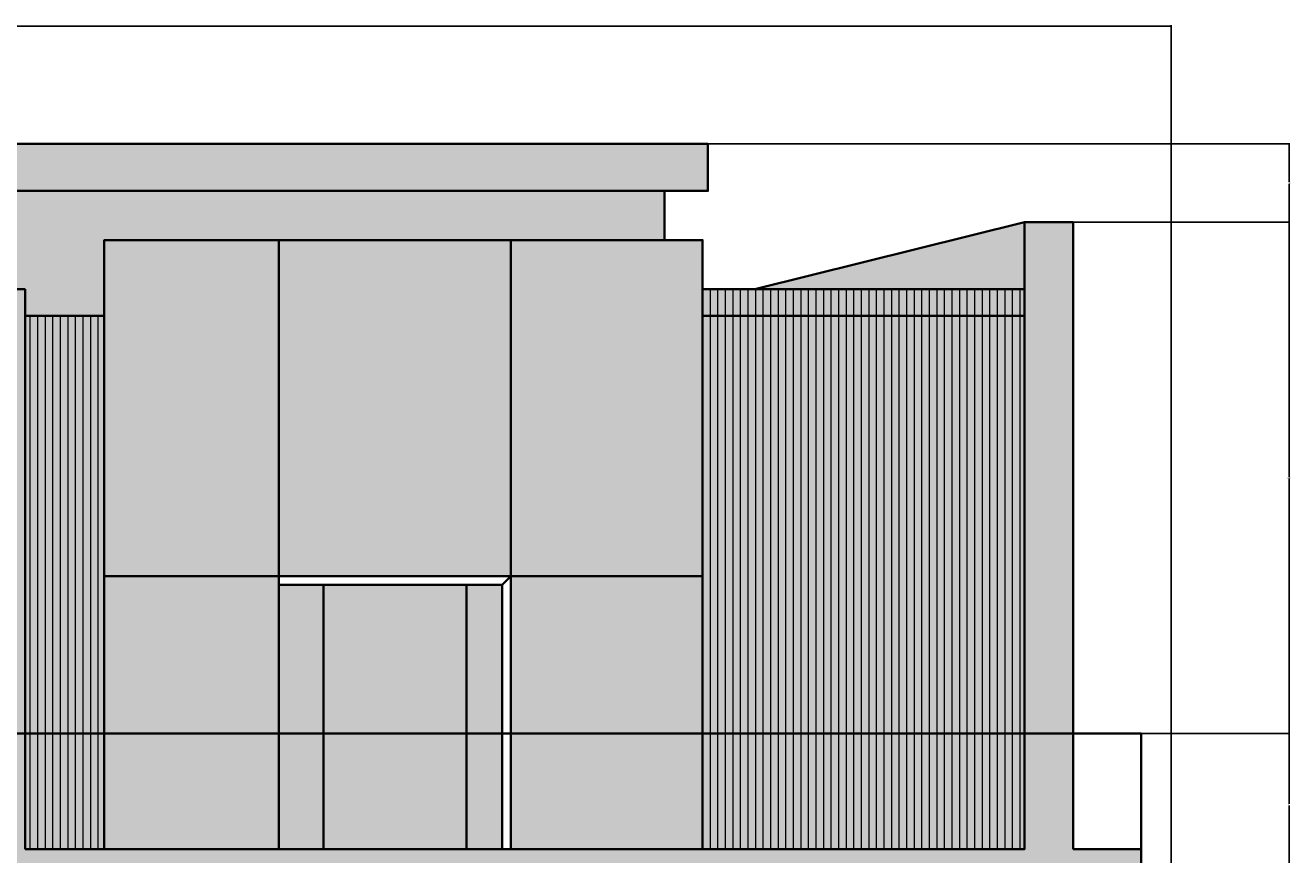
# Model space of a CAD drawing. Units: feet. Extents: x 2651 to 4047, y 949 to 1287.
# Tile 3 of 5: x 2945 to 3230, y 1100 to 1287. Entities that reach past the tile are written whole.
import ezdxf

# ---------------------------------------------------------------- set-up
doc = ezdxf.new("R2010")
doc.units = ezdxf.units.FT
for name, color, linetype, lineweight in [('A-ANNO-DIMS', 2, 'Continuous', 18), ('A-ELEV', 7, 'Continuous', 35), ('A-ELEV-PATT', 8, 'Continuous', 13)]:
    doc.layers.add(name, color=color, linetype=linetype, lineweight=lineweight)
doc.styles.get("Standard").update_dxf_attribs({"font": 'arial.ttf'})
doc.dimstyles.get("Standard").update_dxf_attribs({"dimtxt": 0.18, "dimasz": 0.18, "dimexe": 0.18, "dimexo": 0.0625, "dimgap": 0.09, "dimtad": 0, "dimtih": 1, "dimtoh": 1, "dimdec": 1, "dimzin": 0, "dimdsep": 46, "dimlunit": 3, "dimtxsty": 'Standard', "dimcen": 0.09, "dimadec": 0, "dimazin": 0, "dimtfac": 1, "dimtdec": 1, "dimtofl": 0, "dimtmove": 0, "dimatfit": 3, "dimfxl": 1, "dimtolj": 1, "dimtzin": 0, "dimarcsym": 0})

# ---------------------------------------------------------------- blocks, each defined once
blk = doc.blocks.new('*D7')
at = {"layer": 'A-ANNO-DIMS', "color": 0, "lineweight": -2, "transparency": 16777216}
for p, q in [((2677.56, 975.71), (2677.56, 1287.01)), ((2677.74, 1286.83), (2939.77, 1286.83)), ((3202.59, 1286.83), (2940.56, 1286.83)), ((3202.77, 1095.71), (3202.77, 1287.01))]:
    blk.add_line(p, q, dxfattribs=at)
at = {"layer": 'A-ANNO-DIMS', "color": 0, "transparency": 16777216}
for points in [[(2677.74, 1286.86), (2677.74, 1286.8), (2677.56, 1286.83)], [(3202.59, 1286.86), (3202.59, 1286.8), (3202.77, 1286.83)]]:
    blk.add_solid(points, dxfattribs=at)
at = {"layer": 'Defpoints', "color": 0, "transparency": 16777216}
for p in [(3202.77, 1286.83), (3202.77, 1095.65), (2677.56, 975.65)]:
    blk.add_point(p, dxfattribs=at)
at = {"layer": 'A-ANNO-DIMS', "color": 0, "transparency": 16777216, "insert": (2940.17, 1286.83), "char_height": 0.18, "attachment_point": 5}
blk.add_mtext('\\A1;525.2', dxfattribs=at)
blk = doc.blocks.new('*D8')
at = {"layer": 'A-ANNO-DIMS', "color": 0, "lineweight": -2, "transparency": 16777216}
for p, q in [((3098.48, 1260.33), (2650.88, 1260.33)), ((2651.06, 1260.15), (2651.06, 1118.17)), ((2651.06, 975.83), (2651.06, 1117.81)), ((2677.49, 975.65), (2650.88, 975.65))]:
    blk.add_line(p, q, dxfattribs=at)
at = {"layer": 'A-ANNO-DIMS', "color": 0, "transparency": 16777216}
for points in [[(2651.03, 1260.15), (2651.09, 1260.15), (2651.06, 1260.33)], [(2651.03, 975.83), (2651.09, 975.83), (2651.06, 975.65)]]:
    blk.add_solid(points, dxfattribs=at)
at = {"layer": 'Defpoints', "color": 0, "transparency": 16777216}
for p in [(2651.06, 1260.33), (3098.55, 1260.33), (2677.56, 975.65)]:
    blk.add_point(p, dxfattribs=at)
at = {"layer": 'A-ANNO-DIMS', "color": 0, "transparency": 16777216, "insert": (2651.06, 1117.99), "char_height": 0.18, "attachment_point": 5}
blk.add_mtext('\\A1;284.7', dxfattribs=at)
blk = doc.blocks.new('*D22')
at = {"layer": 'A-ANNO-DIMS', "color": 0, "lineweight": -2, "transparency": 16777216}
for p, q in [((3196.07, 1127.71), (3229.45, 1127.71)), ((3229.27, 1127.53), (3229.27, 1111.86)), ((3229.27, 1095.83), (3229.27, 1111.5)), ((3196.07, 1095.65), (3229.45, 1095.65))]:
    blk.add_line(p, q, dxfattribs=at)
at = {"layer": 'A-ANNO-DIMS', "color": 0, "transparency": 16777216}
for points in [[(3229.24, 1127.53), (3229.3, 1127.53), (3229.27, 1127.71)], [(3229.24, 1095.83), (3229.3, 1095.83), (3229.27, 1095.65)]]:
    blk.add_solid(points, dxfattribs=at)
at = {"layer": 'Defpoints', "color": 0, "transparency": 16777216}
for p in [(3196.01, 1127.71), (3229.27, 1127.71), (3196.01, 1095.65)]:
    blk.add_point(p, dxfattribs=at)
at = {"layer": 'A-ANNO-DIMS', "color": 0, "transparency": 16777216, "insert": (3229.27, 1111.68), "char_height": 0.18, "attachment_point": 5}
blk.add_mtext('\\A1;32.06', dxfattribs=at)
blk = doc.blocks.new('*D23')
at = {"layer": 'A-ANNO-DIMS', "color": 0, "lineweight": -2, "transparency": 16777216}
for p, q in [((3180.76, 1242.69), (3229.45, 1242.69)), ((3229.27, 1242.51), (3229.27, 1185.38)), ((3229.27, 1127.89), (3229.27, 1185.02)), ((3196.07, 1127.71), (3229.45, 1127.71))]:
    blk.add_line(p, q, dxfattribs=at)
at = {"layer": 'A-ANNO-DIMS', "color": 0, "transparency": 16777216}
for points in [[(3229.24, 1242.51), (3229.3, 1242.51), (3229.27, 1242.69)], [(3229.24, 1127.89), (3229.3, 1127.89), (3229.27, 1127.71)]]:
    blk.add_solid(points, dxfattribs=at)
at = {"layer": 'Defpoints', "color": 0, "transparency": 16777216}
for p in [(3180.69, 1242.69), (3229.27, 1242.69), (3196.01, 1127.71)]:
    blk.add_point(p, dxfattribs=at)
at = {"layer": 'A-ANNO-DIMS', "color": 0, "transparency": 16777216, "insert": (3229.27, 1185.2), "char_height": 0.18, "attachment_point": 5}
blk.add_mtext('\\A1;114.98', dxfattribs=at)
blk = doc.blocks.new('*D24')
at = {"layer": 'A-ANNO-DIMS', "color": 0, "lineweight": -2, "transparency": 16777216}
for p, q in [((3098.61, 1260.33), (3229.45, 1260.33)), ((3229.27, 1260.15), (3229.27, 1251.69)), ((3229.27, 1242.87), (3229.27, 1251.33)), ((3180.76, 1242.69), (3229.45, 1242.69))]:
    blk.add_line(p, q, dxfattribs=at)
at = {"layer": 'A-ANNO-DIMS', "color": 0, "transparency": 16777216}
for points in [[(3229.24, 1260.15), (3229.3, 1260.15), (3229.27, 1260.33)], [(3229.24, 1242.87), (3229.3, 1242.87), (3229.27, 1242.69)]]:
    blk.add_solid(points, dxfattribs=at)
at = {"layer": 'Defpoints', "color": 0, "transparency": 16777216}
for p in [(3098.55, 1260.33), (3229.27, 1260.33), (3180.69, 1242.69)]:
    blk.add_point(p, dxfattribs=at)
at = {"layer": 'A-ANNO-DIMS', "color": 0, "transparency": 16777216, "insert": (3229.27, 1251.51), "char_height": 0.18, "attachment_point": 5}
blk.add_mtext('\\A1;17.64', dxfattribs=at)

msp = doc.modelspace()

# ---------------------------------------------------------------- hatches: boundary and pattern name
at = {"layer": 'A-ELEV-PATT'}
msp.add_hatch(color=256, dxfattribs=at).paths.add_polyline_path([(3098.5452, 1260.331), (2886.4328, 1260.331), (2886.4328, 1249.7387), (3098.5452, 1249.7387)])
h = msp.add_hatch(color=256, dxfattribs=at)
h.dxf.hatch_style = 1
h.set_gradient(color1=(199, 200, 202), tint=1, name='HEMISPHERICAL')
h.paths.add_polyline_path([(3169.7582, 1242.6921), (3109.1174, 1227.65), (3169.7582, 1227.65)])
h.paths.add_polyline_path([(3088.7861, 1249.7387), (2896.1919, 1249.7387), (2896.1919, 1227.65), (2944.9934, 1227.65), (2944.9934, 1221.65), (2962.7341, 1221.65), (2962.7341, 1238.6943), (3088.7861, 1238.6943)])
h = msp.add_hatch(color=256, dxfattribs=at)
h.dxf.hatch_style = 1
h.paths.add_polyline_path([(2944.9934, 1227.65), (2896.1919, 1227.65), (2707.3507, 1227.65), (2707.3507, 1221.65), (2938.9934, 1221.65), (2938.9934, 1127.711), (2944.9934, 1127.711), (2944.9934, 1221.65)])
h.paths.add_polyline_path([(2944.9934, 1127.711), (2938.9934, 1127.711), (2938.9934, 1101.65), (2938.9934, 1095.65), (3196.0086, 1095.65), (3196.0086, 1101.65), (3180.6945, 1101.65), (3180.6945, 1127.711), (3169.7582, 1127.711), (3169.7582, 1101.65), (3097.3565, 1101.65), (3002.0224, 1101.65), (2944.9934, 1101.65)])
h.paths.add_polyline_path([(3180.6945, 1242.6921), (3169.7582, 1242.6921), (3169.7582, 1221.65), (3169.7582, 1127.711), (3180.6945, 1127.711)])
h = msp.add_hatch(color=256, dxfattribs=at)
h.set_gradient(color1=(199, 200, 202), color2=(199, 200, 202), tint=1, name='HEMISPHERICAL')
h.paths.add_polyline_path([(2763.5286, 1190.8721), (2719.1033, 1190.8721), (2719.1033, 1152.9072), (2763.5286, 1152.9072)])
h.paths.add_polyline_path([(2838.0977, 1190.8721), (2763.5286, 1190.8721), (2763.5286, 1152.9072), (2838.0977, 1152.9072)])
h.paths.add_polyline_path([(2887.0237, 1190.8721), (2838.0977, 1190.8721), (2838.0977, 1152.9072), (2887.0237, 1152.9072)])
h.paths.add_polyline_path([(2877.0224, 1127.711), (2887.0237, 1127.711), (2887.0237, 1152.9072), (2838.0977, 1152.9072), (2838.0977, 1099.175), (2839.8136, 1099.175), (2839.8136, 1098.3392), (2838.0977, 1098.3392), (2838.0977, 1093.6891), (2839.8136, 1093.6891), (2839.8136, 1092.8533), (2872.1973, 1092.8533), (2872.1973, 1095.65), (2877.0224, 1095.65)])
h.paths.add_polyline_path([(2887.0237, 1127.711), (2877.0224, 1127.711), (2877.0224, 1095.65), (2887.0237, 1095.65)], flags=17)
h.paths.add_polyline_path([(2887.0237, 1084.9772), (2872.1973, 1084.9772), (2872.1973, 1087.7738), (2873.8204, 1087.7738), (2873.8204, 1092.8533), (2872.1973, 1092.8533), (2838.0977, 1092.8533), (2838.0977, 1049.1862), (2887.0237, 1049.1862)])
h.paths.add_polyline_path([(2763.5286, 1152.9072), (2719.1033, 1152.9072), (2719.1033, 1092.8533), (2761.8127, 1092.8533), (2761.8127, 1093.6891), (2763.5286, 1093.6891), (2763.5286, 1098.3392), (2761.8127, 1098.3392), (2761.8127, 1099.175), (2763.5286, 1099.175)])
h.paths.add_polyline_path([(2763.5286, 1092.8533), (2719.1033, 1092.8533), (2719.1033, 1049.1862), (2763.5286, 1049.1862), (2763.5286, 1072.7574)])
h.paths.add_polyline_path([(2838.0977, 1152.9072), (2763.5286, 1152.9072), (2763.5286, 1148.4143), (2838.0977, 1148.4143)])
h.paths.add_polyline_path([(2838.0977, 1092.8533), (2763.5286, 1092.8533), (2763.5286, 1072.7574), (2838.0977, 1072.7574)])
h.paths.add_polyline_path([(2883.0637, 1047.7503), (2677.5561, 1047.7503), (2677.5561, 1035.7503), (2871.0637, 1035.7503), (2871.0637, 975.65), (2883.0637, 975.65)])
h.paths.add_polyline_path([(2911.0266, 1047.7503), (2898.171, 1047.7503), (2898.171, 975.65), (2911.0266, 975.65)])
h.paths.add_polyline_path([(2932.4585, 1047.7503), (2919.6029, 1047.7503), (2919.6029, 975.65), (2932.4585, 975.65)])
h.paths.add_polyline_path([(2953.8904, 1047.7503), (2941.0349, 1047.7503), (2941.0349, 975.65), (2953.8904, 975.65)])
h.paths.add_polyline_path([(2985.9915, 1047.7503), (2962.4668, 1047.7503), (2962.4668, 975.65), (2975.3223, 975.65), (2985.9915, 975.65)])
h.paths.add_polyline_path([(3097.3565, 1221.65), (3097.3565, 1238.6943), (3054.2372, 1238.6943), (3054.2372, 1163.1131), (3097.3565, 1163.1131)])
h.paths.add_polyline_path([(3002.0224, 1238.6943), (2962.7341, 1238.6943), (2962.7341, 1163.1131), (3002.0224, 1163.1131)])
h.paths.add_polyline_path([(3054.2372, 1238.6943), (3002.0224, 1238.6943), (3002.0224, 1163.1131), (3054.2372, 1163.1131)])
h.paths.add_polyline_path([(3002.0224, 1163.1131), (2962.7341, 1163.1131), (2962.7341, 1127.711), (3002.0224, 1127.711)])
h.paths.add_polyline_path([(3002.0224, 1127.711), (2962.7341, 1127.711), (2962.7341, 1101.65), (3002.0224, 1101.65)])
h.paths.add_polyline_path([(3097.3565, 1163.1131), (3054.2372, 1163.1131), (3054.2372, 1127.711), (3097.3565, 1127.711)])
h.paths.add_polyline_path([(3097.3565, 1127.711), (3054.2372, 1127.711), (3054.2372, 1101.65), (3097.3565, 1101.65)])
h = msp.add_hatch(dxfattribs=at)
h.set_pattern_fill('AR-SAND', color=256, scale=0.09, style=0)
h.set_pattern_definition([(37.5, (-817.72, 3e-12), (-0.1440028, 4.404719), [0, -3.47472, 0, -3.8862, 0, -3.71475]), (7.5, (-817.72, 3e-12), (4.0457095, 6.451426), [0, -1.87452, 0, -3.13182, 0, -1.20015]), (327.5, (-820.5318, 3e-12), (7.1189313, 0.0129347), [0, -1.143, 0, -4.1148, 0, -5.3721]), (317.5, (-820.532, 3e-12), (6.872008, 2.006364), [0, -0.5715, 0, -2.69748, 0, -3.0861])])
h.paths.add_polyline_path([(3002.0224, 1238.6943), (2962.7341, 1238.6943), (2962.7341, 1163.1131), (3002.0224, 1163.1131)])
h.paths.add_polyline_path([(3054.2372, 1238.6943), (3002.0224, 1238.6943), (3002.0224, 1163.1131), (3054.2372, 1163.1131)])
h.paths.add_polyline_path([(3097.3565, 1221.65), (3097.3565, 1238.6943), (3054.2372, 1238.6943), (3054.2372, 1163.1131), (3097.3565, 1163.1131)])
h.paths.add_polyline_path([(3097.3565, 1163.1131), (3054.2372, 1163.1131), (3054.2372, 1127.711), (3097.3565, 1127.711)])
h.paths.add_polyline_path([(3097.3565, 1127.711), (3054.2372, 1127.711), (3054.2372, 1101.65), (3097.3565, 1101.65)])
h.paths.add_polyline_path([(3002.0224, 1127.711), (2962.7341, 1127.711), (2962.7341, 1101.65), (3002.0224, 1101.65)])
h.paths.add_polyline_path([(3002.0224, 1163.1131), (2962.7341, 1163.1131), (2962.7341, 1127.711), (3002.0224, 1127.711)])
h = msp.add_hatch(color=256, dxfattribs=at)
h.set_gradient(color1=(168, 95, 18), color2=(168, 95, 18), tint=1, name='CURVED')
h.paths.add_polyline_path([(2938.9934, 1207.954), (2732.0644, 1207.954), (2732.0644, 1190.8721), (2887.0237, 1190.8721), (2887.0237, 1127.711), (2938.9934, 1127.711)])
h.paths.add_polyline_path([(2938.9934, 1221.65), (2707.3507, 1221.65), (2732.0644, 1207.954), (2938.9934, 1207.954)])
h.paths.add_polyline_path([(3169.7582, 1221.65), (3097.3565, 1221.65), (3097.3565, 1127.711), (3169.7582, 1127.711)])
h.paths.add_polyline_path([(2962.7341, 1221.65), (2944.9934, 1221.65), (2944.9934, 1127.711), (2962.7341, 1127.711)])
h.paths.add_polyline_path([(3169.7582, 1227.65), (3097.3565, 1227.65), (3097.3565, 1221.65), (3169.7582, 1221.65)])
h.paths.add_polyline_path([(3169.7582, 1127.711), (3097.3565, 1127.711), (3097.3565, 1101.65), (3169.7582, 1101.65)])
h.paths.add_polyline_path([(2962.7341, 1127.711), (2944.9934, 1127.711), (2944.9934, 1101.65), (2962.7341, 1101.65)])
h.paths.add_polyline_path([(2938.9934, 1127.711), (2887.0237, 1127.711), (2887.0237, 1095.65), (2938.9934, 1095.65), (2938.9934, 1101.65)])
h.paths.add_polyline_path([(2944.9934, 1084.9772), (2887.0237, 1084.9772), (2887.0237, 1049.1862), (2883.0637, 1049.1862), (2883.0637, 1047.7503), (2883.0637, 1035.7503), (2898.171, 1035.7503), (2898.171, 1047.7503), (2898.171, 1049.1862), (2911.0266, 1049.1862), (2911.0266, 1035.7503), (2919.6029, 1035.7503), (2919.6029, 1047.7503), (2919.6029, 1049.1862), (2932.4585, 1049.1862), (2932.4585, 1035.7503), (2941.0349, 1035.7503), (2941.0349, 1047.7503), (2941.0349, 1049.1862), (2944.9934, 1049.1862)])
h = msp.add_hatch(dxfattribs=at)
h.set_pattern_fill('_USER', color=256, scale=1.7, angle=90, style=0, pattern_type=0)
h.set_pattern_definition([(90, (0, 0), (-1.7, 1e-16), [])])
h.paths.add_polyline_path([(2938.9934, 1207.954), (2732.0644, 1207.954), (2732.0644, 1190.8721), (2887.0237, 1190.8721), (2887.0237, 1127.711), (2938.9934, 1127.711)])
h.paths.add_polyline_path([(2938.9934, 1221.65), (2707.3507, 1221.65), (2732.0644, 1207.954), (2938.9934, 1207.954)])
h.paths.add_polyline_path([(2938.9934, 1127.711), (2887.0237, 1127.711), (2887.0237, 1095.65), (2938.9934, 1095.65), (2938.9934, 1101.65)])
h.paths.add_polyline_path([(2962.7341, 1221.65), (2944.9934, 1221.65), (2944.9934, 1127.711), (2962.7341, 1127.711)])
h.paths.add_polyline_path([(2962.7341, 1127.711), (2944.9934, 1127.711), (2944.9934, 1101.65), (2962.7341, 1101.65)])
h.paths.add_polyline_path([(3169.7582, 1221.65), (3097.3565, 1221.65), (3097.3565, 1127.711), (3169.7582, 1127.711)])
h.paths.add_polyline_path([(3169.7582, 1227.65), (3097.3565, 1227.65), (3097.3565, 1221.65), (3169.7582, 1221.65)])
h.paths.add_polyline_path([(3169.7582, 1127.711), (3097.3565, 1127.711), (3097.3565, 1101.65), (3169.7582, 1101.65)])
h.paths.add_polyline_path([(2944.9934, 1084.9772), (2887.0237, 1084.9772), (2887.0237, 1049.1862), (2883.0637, 1049.1862), (2883.0637, 1047.7503), (2883.0637, 1035.7503), (2898.171, 1035.7503), (2898.171, 1047.7503), (2898.171, 1049.1862), (2911.0266, 1049.1862), (2911.0266, 1035.7503), (2919.6029, 1035.7503), (2919.6029, 1047.7503), (2919.6029, 1049.1862), (2932.4585, 1049.1862), (2932.4585, 1035.7503), (2941.0349, 1035.7503), (2941.0349, 1047.7503), (2941.0349, 1049.1862), (2944.9934, 1049.1862)])
h = msp.add_hatch(color=256, dxfattribs=at)
h.set_gradient(color1=(194, 211, 228), color2=(194, 211, 228), name='HEMISPHERICAL')
h.paths.add_polyline_path([(3012.0516, 1161.1131), (3002.0224, 1161.1131), (3002.0224, 1127.711), (3012.0516, 1127.711)])
h.paths.add_polyline_path([(3012.0516, 1127.711), (3002.0224, 1127.711), (3002.0224, 1101.65), (3012.0516, 1101.65)])
h.paths.add_polyline_path([(3044.208, 1161.1131), (3012.0516, 1161.1131), (3012.0516, 1127.711), (3044.208, 1127.711)])
h.paths.add_polyline_path([(3044.208, 1127.711), (3012.0516, 1127.711), (3012.0516, 1101.65), (3044.208, 1101.65)])
h.paths.add_polyline_path([(3052.2372, 1161.1131), (3044.208, 1161.1131), (3044.208, 1127.711), (3052.2372, 1127.711)])
h.paths.add_polyline_path([(3052.2372, 1127.711), (3044.208, 1127.711), (3044.208, 1101.65), (3052.2372, 1101.65)])

# ---------------------------------------------------------------- linework, layer by layer
at = {"layer": 'A-ELEV'}
for p, q in [((3169.7582, 1242.6921), (3109.1174, 1227.65)), ((3169.7582, 1242.6921), (3109.1174, 1227.65)), ((3002.0224, 1238.6943), (3002.0224, 1101.65)), ((3002.0224, 1238.6943), (3002.0224, 1101.65)), ((3054.2372, 1238.6943), (3054.2372, 1101.65)), ((3054.2372, 1238.6943), (3054.2372, 1101.65)), ((2944.9934, 1221.65), (2944.9934, 1227.65)), ((2944.9934, 1221.65), (2944.9934, 1227.65)), ((3097.3565, 1227.65), (3169.7582, 1227.65)), ((3097.3565, 1227.65), (3169.7582, 1227.65)), ((2962.7341, 1221.65), (2944.9934, 1221.65)), ((2962.7341, 1221.65), (2944.9934, 1221.65)), ((3169.7582, 1221.65), (3097.3565, 1221.65)), ((3169.7582, 1221.65), (3097.3565, 1221.65)), ((2962.7341, 1163.1131), (3097.3565, 1163.1131)), ((2962.7341, 1163.1131), (3097.3565, 1163.1131)), ((3052.2372, 1161.1131), (3054.2372, 1163.1131)), ((3052.2372, 1161.1131), (3054.2372, 1163.1131)), ((3012.0516, 1161.1131), (3012.0516, 1101.65)), ((3012.0516, 1161.1131), (3012.0516, 1101.65)), ((3044.208, 1161.1131), (3044.208, 1101.65)), ((3044.208, 1161.1131), (3044.208, 1101.65)), ((3196.0086, 1127.711), (2877.0224, 1127.711)), ((3196.0086, 1127.711), (2877.0224, 1127.711)), ((3196.0086, 1127.711), (3196.0086, 1095.65)), ((3196.0086, 1127.711), (3196.0086, 1095.65)), ((2944.9934, 1101.65), (3169.7582, 1101.65)), ((2944.9934, 1101.65), (3169.7582, 1101.65)), ((3180.6945, 1101.65), (3196.0086, 1101.65)), ((3180.6945, 1101.65), (3196.0086, 1101.65))]:
    msp.add_line(p, q, dxfattribs=at)
for points in [[(2886.4328, 1249.7387), (3098.5452, 1249.7387), (3098.5452, 1260.331), (2886.4328, 1260.331)], [(2886.4328, 1249.7387), (3098.5452, 1249.7387), (3098.5452, 1260.331), (2886.4328, 1260.331)], [(3097.3565, 1101.65), (3169.7582, 1101.65), (3169.7582, 1221.65), (3097.3565, 1221.65)], [(3097.3565, 1101.65), (3169.7582, 1101.65), (3169.7582, 1221.65), (3097.3565, 1221.65)], [(3054.2372, 1101.65), (3002.0224, 1101.65), (3002.0224, 1163.1131), (3054.2372, 1163.1131)], [(3054.2372, 1101.65), (3002.0224, 1101.65), (3002.0224, 1163.1131), (3054.2372, 1163.1131)]]:
    msp.add_lwpolyline(points, close=True, dxfattribs=at)
for points in [[(3088.7861, 1238.6943), (3088.7861, 1249.7387), (2896.1919, 1249.7387), (2896.1919, 1227.65), (2944.9934, 1227.65)], [(3088.7861, 1238.6943), (3088.7861, 1249.7387), (2896.1919, 1249.7387), (2896.1919, 1227.65), (2944.9934, 1227.65)], [(3180.6945, 1101.65), (3180.6945, 1242.6921), (3169.7582, 1242.6921), (3169.7582, 1221.65)], [(3180.6945, 1101.65), (3180.6945, 1242.6921), (3169.7582, 1242.6921), (3169.7582, 1221.65)], [(3002.0224, 1101.65), (3097.3565, 1101.65), (3097.3565, 1238.6943), (2962.7341, 1238.6943), (2962.7341, 1101.65)], [(3002.0224, 1101.65), (3097.3565, 1101.65), (3097.3565, 1238.6943), (2962.7341, 1238.6943), (2962.7341, 1101.65)], [(2944.9934, 1221.65), (2944.9934, 1101.65)], [(2944.9934, 1221.65), (2944.9934, 1101.65)], [(3002.0224, 1161.1131), (3052.2372, 1161.1131), (3052.2372, 1101.65)], [(3002.0224, 1161.1131), (3052.2372, 1161.1131), (3052.2372, 1101.65)]]:
    msp.add_lwpolyline(points, dxfattribs=at)

# ---------------------------------------------------------------- dimensions: what is measured, and where the dimension line sits
at = {"layer": 'A-ANNO-DIMS'}
dim = msp.add_linear_dim(base=(3202.774, 1286.831), p1=(2677.5561, 975.65), p2=(3202.774, 1095.65), dimstyle='Standard', override={"dimdec": 1, "dimlfac": 1, "dimrnd": 0, "dimzin": 0, "dimdsep": 46, "dimlunit": 2}, dxfattribs=at)
dim.commit()
dim.dimension.update_dxf_attribs({"geometry": '*D7', "text_midpoint": (2940.1651, 1286.831)})
for base, p1, p2, override, picture, middle in [((2651.0561, 1260.331), (2677.5561, 975.65), (3098.5452, 1260.331), {"dimdec": 1, "dimlfac": 1, "dimrnd": 0, "dimzin": 0, "dimdsep": 46, "dimlunit": 2}, '*D8', (2651.0561, 1117.9905)), ((3229.274, 1260.331), (3180.6945, 1242.6921), (3098.5452, 1260.331), {"dimdec": 2, "dimlfac": 1, "dimrnd": 0, "dimzin": 0, "dimdsep": 46, "dimlunit": 2}, '*D24', (3229.274, 1251.5116)), ((3229.274, 1242.6921), (3196.0086, 1127.711), (3180.6945, 1242.6921), {"dimdec": 2, "dimlfac": 1, "dimrnd": 0, "dimzin": 0, "dimdsep": 46, "dimlunit": 2}, '*D23', (3229.274, 1185.2016)), ((3229.274, 1127.711), (3196.0086, 1095.65), (3196.0086, 1127.711), {"dimdec": 2, "dimlfac": 1, "dimrnd": 0, "dimzin": 0, "dimdsep": 46, "dimlunit": 2}, '*D22', (3229.274, 1111.6805))]:
    dim = msp.add_linear_dim(base=base, p1=p1, p2=p2, angle=90, dimstyle='Standard', override=override, dxfattribs=at)
    dim.commit()
    dim.dimension.update_dxf_attribs({"geometry": picture, "text_midpoint": middle})

doc.saveas('drawing.dxf')
